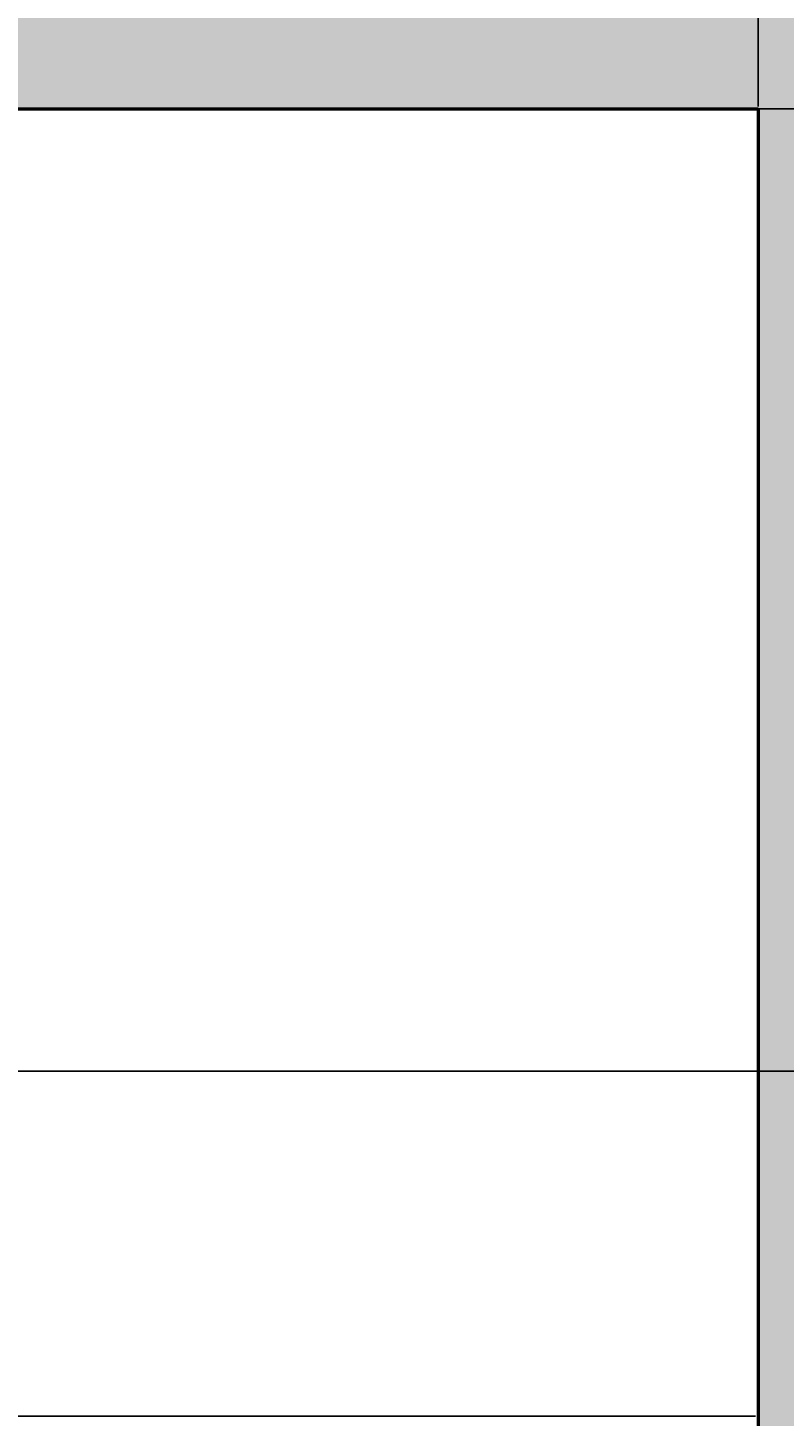
# Model space of a CAD drawing. Units: inches. Extents: x 2231 to 2461, y 2045 to 2455.
# Tile 34 of 95: x 2415 to 2433, y 2151 to 2185. Entities that reach past the tile are written whole.
import ezdxf

# ---------------------------------------------------------------- set-up
doc = ezdxf.new("R2010")
doc.units = ezdxf.units.IN
doc.layers.add('A-ANNO-DIMS', color=2, linetype='Continuous', lineweight=18)
doc.layers.add('A-WALL', color=7, linetype='Continuous', lineweight=50)
doc.layers.add('A-WALL-PATT', color=18, linetype='Continuous', lineweight=13, true_color=0x000000)
doc.styles.get("Standard").update_dxf_attribs({"font": 'arial.ttf'})
doc.dimstyles.get("Standard").update_dxf_attribs({"dimtxt": 0.18, "dimasz": 0.18, "dimexe": 0.18, "dimexo": 0.0625, "dimgap": 0.09, "dimtad": 0, "dimtih": 1, "dimtoh": 1, "dimdec": 4, "dimzin": 0, "dimdsep": 46, "dimtxsty": 'Standard', "dimcen": 0.09, "dimadec": 0, "dimazin": 0, "dimtfac": 1, "dimtdec": 4, "dimtofl": 0, "dimtmove": 0, "dimatfit": 3, "dimfxl": 1, "dimtolj": 1, "dimtzin": 0, "dimarcsym": 0})

# ---------------------------------------------------------------- blocks, each defined once
blk = doc.blocks.new('*D41')
at = {"layer": 'A-ANNO-DIMS', "color": 0, "lineweight": -2, "transparency": 16777216}
for p, q in [((2432.856, 2182.833), (2460.606, 2182.833)), ((2460.426, 2182.653), (2460.426, 2128.015)), ((2460.426, 2073.013), (2460.426, 2127.651)), ((2432.856, 2072.833), (2460.606, 2072.833))]:
    blk.add_line(p, q, dxfattribs=at)
at = {"layer": 'A-ANNO-DIMS', "color": 0, "transparency": 16777216}
for points in [[(2460.396, 2182.653), (2460.456, 2182.653), (2460.426, 2182.833)], [(2460.396, 2073.013), (2460.456, 2073.013), (2460.426, 2072.833)]]:
    blk.add_solid(points, dxfattribs=at)
at = {"layer": 'Defpoints', "color": 0, "transparency": 16777216}
for p in [(2432.794, 2182.833), (2460.426, 2182.833), (2432.794, 2072.833)]:
    blk.add_point(p, dxfattribs=at)
at = {"layer": 'A-ANNO-DIMS', "color": 0, "transparency": 16777216, "insert": (2460.426, 2127.833), "char_height": 0.18, "attachment_point": 5}
blk.add_mtext('\\A1;110', dxfattribs=at)
blk = doc.blocks.new('*D59')
at = {"layer": 'A-ANNO-DIMS', "color": 0, "lineweight": -2, "transparency": 16777216}
for p, q in [((2408.794, 2182.895), (2408.794, 2454.645)), ((2432.794, 2182.895), (2432.794, 2454.645)), ((2408.974, 2454.465), (2420.573, 2454.465)), ((2432.614, 2454.465), (2421.014, 2454.465))]:
    blk.add_line(p, q, dxfattribs=at)
at = {"layer": 'A-ANNO-DIMS', "color": 0, "transparency": 16777216}
for points in [[(2408.974, 2454.495), (2408.974, 2454.435), (2408.794, 2454.465)], [(2432.614, 2454.495), (2432.614, 2454.435), (2432.794, 2454.465)]]:
    blk.add_solid(points, dxfattribs=at)
at = {"layer": 'Defpoints', "color": 0, "transparency": 16777216}
for p in [(2432.794, 2454.465), (2408.794, 2182.833), (2432.794, 2182.833)]:
    blk.add_point(p, dxfattribs=at)
at = {"layer": 'A-ANNO-DIMS', "color": 0, "transparency": 16777216, "insert": (2420.794, 2454.465), "char_height": 0.18, "attachment_point": 5}
blk.add_mtext('\\A1;24', dxfattribs=at)
blk = doc.blocks.new('*D60')
at = {"layer": 'A-ANNO-DIMS', "color": 0, "lineweight": -2, "transparency": 16777216}
for p, q in [((2432.731, 2182.833), (2230.981, 2182.833)), ((2231.161, 2182.653), (2231.161, 2166.906)), ((2231.161, 2150.795), (2231.161, 2166.542)), ((2432.731, 2150.615), (2230.981, 2150.615))]:
    blk.add_line(p, q, dxfattribs=at)
at = {"layer": 'A-ANNO-DIMS', "color": 0, "transparency": 16777216}
for points in [[(2231.131, 2182.653), (2231.191, 2182.653), (2231.161, 2182.833)], [(2231.131, 2150.795), (2231.191, 2150.795), (2231.161, 2150.615)]]:
    blk.add_solid(points, dxfattribs=at)
at = {"layer": 'Defpoints', "color": 0, "transparency": 16777216}
for p in [(2231.161, 2182.833), (2432.794, 2182.833), (2432.794, 2150.615)]:
    blk.add_point(p, dxfattribs=at)
at = {"layer": 'A-ANNO-DIMS', "color": 0, "transparency": 16777216, "insert": (2231.161, 2166.724), "char_height": 0.18, "attachment_point": 5}
blk.add_mtext('\\A1;32.22', dxfattribs=at)
blk = doc.blocks.new('*D73')
at = {"layer": 'A-ANNO-DIMS', "color": 0, "lineweight": -2, "transparency": 16777216}
for p, q in [((2334.856, 2182.833), (2460.606, 2182.833)), ((2460.426, 2182.653), (2460.426, 2171.156)), ((2460.426, 2159.295), (2460.426, 2170.792)), ((2353.872, 2159.115), (2460.606, 2159.115))]:
    blk.add_line(p, q, dxfattribs=at)
at = {"layer": 'A-ANNO-DIMS', "color": 0, "transparency": 16777216}
for points in [[(2460.396, 2182.653), (2460.456, 2182.653), (2460.426, 2182.833)], [(2460.396, 2159.295), (2460.456, 2159.295), (2460.426, 2159.115)]]:
    blk.add_solid(points, dxfattribs=at)
at = {"layer": 'Defpoints', "color": 0, "transparency": 16777216}
for p in [(2334.794, 2182.833), (2460.426, 2182.833), (2353.809, 2159.115)]:
    blk.add_point(p, dxfattribs=at)
at = {"layer": 'A-ANNO-DIMS', "color": 0, "transparency": 16777216, "insert": (2460.426, 2170.974), "char_height": 0.18, "attachment_point": 5}
blk.add_mtext('\\A1;23.717', dxfattribs=at)

msp = doc.modelspace()

# ---------------------------------------------------------------- hatches: boundary and pattern name
at = {"layer": 'A-WALL-PATT'}
h = msp.add_hatch(color=256, dxfattribs=at)
h.dxf.hatch_style = 1
h.paths.add_polyline_path([(2441.7935, 2269.1535), (2432.7935, 2269.1535), (2432.7935, 2186.8328), (2396.7935, 2186.8328), (2396.7935, 2286.8328), (2394.7935, 2286.8328), (2394.7935, 2186.8328), (2334.7935, 2186.8328), (2334.7935, 2182.8328), (2432.7935, 2182.8328), (2432.7935, 2072.8328), (2416.6639, 2072.8328), (2416.6639, 2063.8328), (2441.7935, 2063.8328)])
h.paths.add_polyline_path([(2368.6639, 2072.8328), (2367.04, 2072.8328), (2330.7942, 2072.8328), (2330.7397, 2063.8328), (2368.6639, 2063.8328)])
h.paths.add_polyline_path([(2300.7392, 2068.3328), (2300.7392, 2072.8328), (2298.7935, 2072.8328), (2294.7935, 2072.8328), (2258.7935, 2072.8328), (2258.7935, 2120.8328), (2294.7935, 2120.8328), (2298.7935, 2120.8328), (2298.7935, 2128.8328), (2294.7935, 2128.8328), (2294.7935, 2124.8328), (2258.7935, 2124.8328), (2258.7935, 2182.8328), (2294.7935, 2182.8328), (2294.7935, 2174.8328), (2298.7935, 2174.8328), (2298.7935, 2182.8328), (2304.7935, 2182.8328), (2304.7935, 2186.8328), (2258.7935, 2186.8328), (2258.7935, 2221.999), (2249.7935, 2221.999), (2249.7935, 2063.8328), (2300.7392, 2063.8328)])
h.paths.add_polyline_path([(2391.9338, 2435.8328), (2333.82, 2435.8328), (2333.82, 2426.8328), (2368.7935, 2426.8328), (2368.7935, 2374.9508), (2368.7935, 2370.8328), (2372.3935, 2370.8328), (2372.7935, 2370.8328), (2372.7935, 2426.8328), (2391.9338, 2426.8328)])
h.paths.add_polyline_path([(2441.7935, 2435.8328), (2415.9338, 2435.8328), (2415.9338, 2426.8328), (2432.7935, 2426.8328), (2432.7935, 2334.8328), (2372.7935, 2334.8328), (2372.7935, 2346.8328), (2368.7935, 2346.8328), (2368.7935, 2306.8328), (2360.7935, 2306.8328), (2360.7935, 2302.8328), (2368.7935, 2302.8328), (2372.7935, 2302.8328), (2372.7935, 2330.8328), (2432.7935, 2330.8328), (2432.7935, 2317.1535), (2441.7935, 2317.1535)])
h.paths.add_polyline_path([(2285.82, 2435.8328), (2249.7935, 2435.8328), (2249.7935, 2269.999), (2258.7935, 2269.999), (2258.7935, 2302.8328), (2318.8168, 2302.8328), (2330.7935, 2302.8328), (2330.7935, 2306.8328), (2258.7935, 2306.8328), (2258.7935, 2426.8328), (2285.82, 2426.8328)])

# ---------------------------------------------------------------- linework, layer by layer
at = {"layer": 'A-WALL'}
for p, q in [((2334.7935, 2182.8328), (2432.7935, 2182.8328)), ((2432.7935, 2182.8328), (2432.7935, 2072.8328))]:
    msp.add_line(p, q, dxfattribs=at)

# ---------------------------------------------------------------- dimensions: what is measured, and where the dimension line sits
at = {"layer": 'A-ANNO-DIMS'}
dim = msp.add_linear_dim(base=(2432.7935, 2454.4653), p1=(2408.7935, 2182.8328), p2=(2432.7935, 2182.8328), dimstyle='Standard', override={"dimdec": 0, "dimlfac": 1, "dimrnd": 0, "dimzin": 0, "dimdsep": 46, "dimlunit": 2}, dxfattribs=at)
dim.commit()
dim.dimension.update_dxf_attribs({"geometry": '*D59', "text_midpoint": (2420.7935, 2454.4653)})
for base, p1, p2, override, picture, middle in [((2231.161, 2182.8328), (2432.7935, 2150.6145), (2432.7935, 2182.8328), {"dimdec": 2, "dimlfac": 1, "dimrnd": 0, "dimzin": 0, "dimdsep": 46, "dimlunit": 2}, '*D60', (2231.161, 2166.7237)), ((2460.426, 2182.8328), (2353.8091, 2159.1154), (2334.7935, 2182.8328), {"dimdec": 3, "dimlfac": 1, "dimrnd": 0, "dimzin": 0, "dimdsep": 46, "dimlunit": 2}, '*D73', (2460.426, 2170.9741)), ((2460.426, 2182.8328), (2432.7935, 2072.8328), (2432.7935, 2182.8328), {"dimdec": 0, "dimlfac": 1, "dimrnd": 0, "dimzin": 0, "dimdsep": 46, "dimlunit": 2}, '*D41', (2460.426, 2127.8328))]:
    dim = msp.add_linear_dim(base=base, p1=p1, p2=p2, angle=90, dimstyle='Standard', override=override, dxfattribs=at)
    dim.commit()
    dim.dimension.update_dxf_attribs({"geometry": picture, "text_midpoint": middle})

doc.saveas('drawing.dxf')
